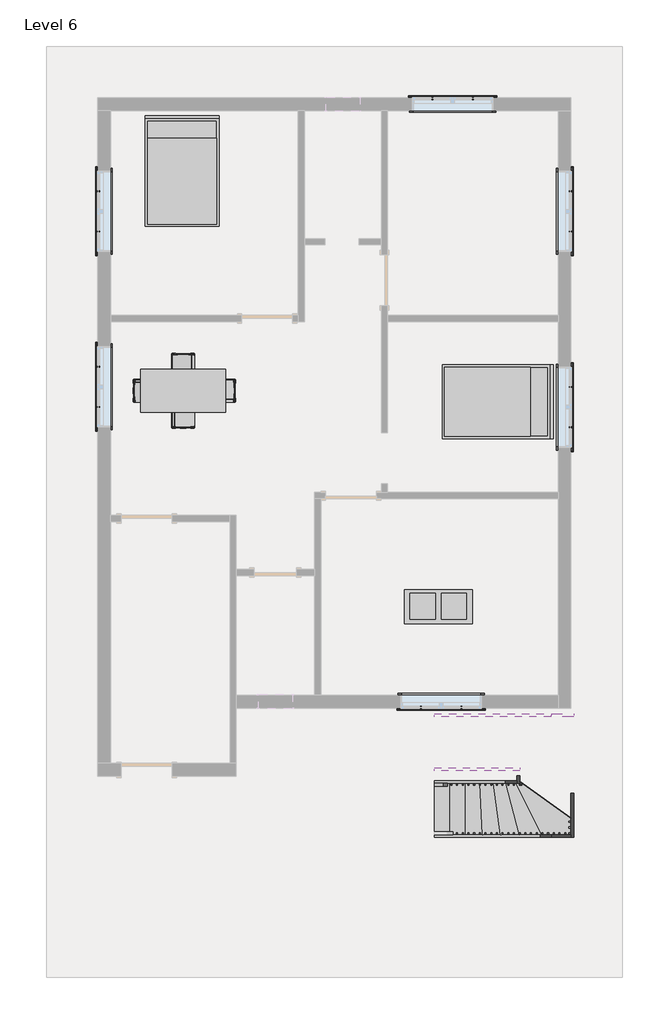
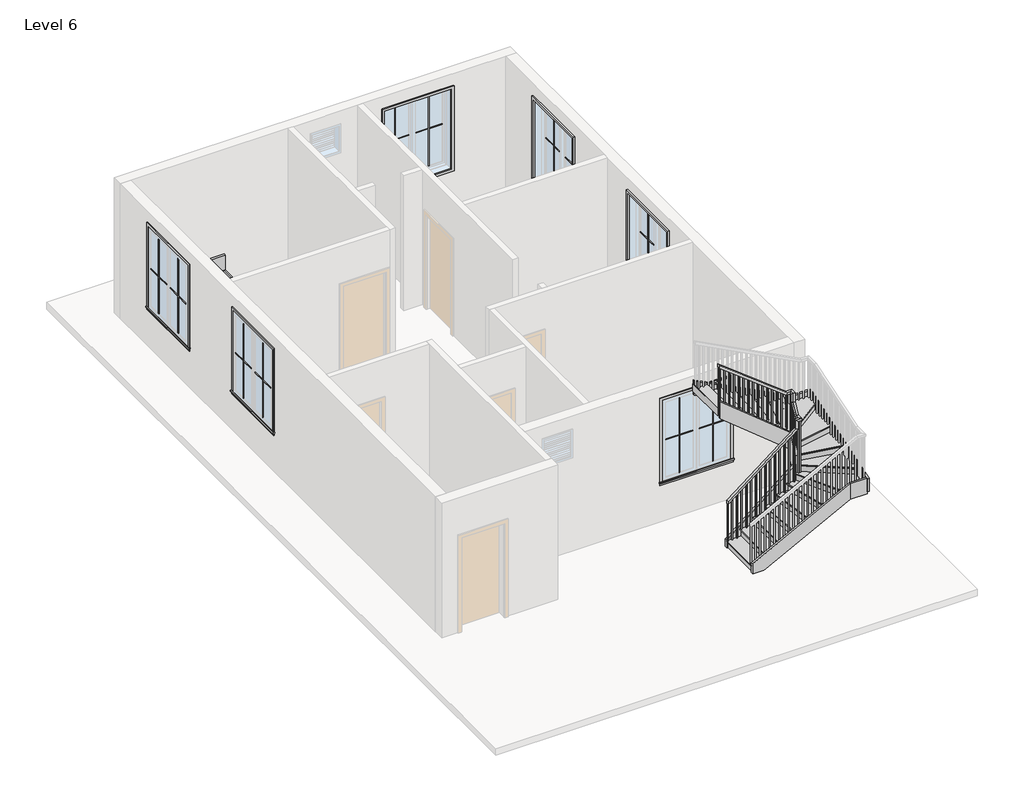
# One storey, part 3 of 3: 25 proxies, 8 members, 3 furniture elements, 1 railing, 1 stair flight.
"""IFC4 building model written with IfcOpenShell, lengths in millimetres."""

from ifc_helpers import new_model, si_unit, frame, origin, place, context, project, spatial, polyline, outline, extrude, faceted_brep, transform, mapped, element, save
from components import muntin_pattern_2x2_muntin_pattern_2x2_bff912c5, muntin_pattern_2x2_muntin_pattern_2x2_c2194282, trim_window_exterior_flat_with_sill_e04b3088, trim_window_interior_flat_picture_frame_2a7685fe, coffee_table_with_brass_mullions_11320_coffee_table_with_5962bef7, bed_17739_bed_17739_15c61121, dining_table_w_chairs_11374_0cdfc61b, stair_flight_916a27e3

model = new_model("IFC4")

# Units and contexts
model_context = context("Model", 3, world=origin())
ifc_project = project(units=[si_unit("LENGTHUNIT", "METRE", prefix="MILLI")], contexts=[model_context])

# Site, building, storey
site = spatial("IfcSite", under=ifc_project)
building = spatial("IfcBuilding", under=site)
storey = spatial("IfcBuildingStorey", under=building, Name="Level 6", Elevation=12801.6)

# Proxies
placement = place(None, origin())
muntin_pattern_2x2_muntin_pattern_2x2_shape = muntin_pattern_2x2_muntin_pattern_2x2_bff912c5(model_context)
element("IfcBuildingElementProxy", 1, Name="Muntin Pattern_2x2 : Muntin Pattern_2x2", ObjectType="Muntin Pattern_2x2 : Muntin Pattern_2x2", at=placement, inside=storey, context=model_context, shape_type="MappedRepresentation", body=[
    mapped(muntin_pattern_2x2_muntin_pattern_2x2_shape, transform((2964.3605034, 427.8534591, 13785.85), x_axis=(0.0, -1.0, 0.0), y_axis=(1.0, 0.0, 0.0), z_axis=(0.0, 0.0, 1.0))),
])
element("IfcBuildingElementProxy", 2, Name="Muntin Pattern_2x2 : Muntin Pattern_2x2", ObjectType="Muntin Pattern_2x2 : Muntin Pattern_2x2", at=placement, inside=storey, context=model_context, shape_type="MappedRepresentation", body=[
    mapped(muntin_pattern_2x2_muntin_pattern_2x2_shape, transform((2964.3605034, 3923.5284591, 13785.85), x_axis=(0.0, -1.0, 0.0), y_axis=(1.0, 0.0, 0.0), z_axis=(0.0, 0.0, 1.0))),
])
element("IfcBuildingElementProxy", 3, Name="Muntin Pattern_2x2 : Muntin Pattern_2x2", ObjectType="Muntin Pattern_2x2 : Muntin Pattern_2x2", at=placement, inside=storey, context=model_context, shape_type="MappedRepresentation", body=[
    mapped(muntin_pattern_2x2_muntin_pattern_2x2_shape, transform((498.9730034, 5582.4659591, 13785.85), x_axis=(1.0, 0.0, 0.0), y_axis=(0.0, 1.0, 0.0), z_axis=(0.0, 0.0, 1.0))),
])
element("IfcBuildingElementProxy", 4, Name="Muntin Pattern_2x2 : Muntin Pattern_2x2", ObjectType="Muntin Pattern_2x2 : Muntin Pattern_2x2", at=placement, inside=storey, context=model_context, shape_type="MappedRepresentation", body=[
    mapped(muntin_pattern_2x2_muntin_pattern_2x2_shape, transform((-5474.7894966, 3202.8034591, 13785.85), x_axis=(0.0, 1.0, 0.0), y_axis=(-1.0, 0.0, 0.0), z_axis=(0.0, 0.0, 1.0))),
])
element("IfcBuildingElementProxy", 5, Name="Muntin Pattern_2x2 : Muntin Pattern_2x2", ObjectType="Muntin Pattern_2x2 : Muntin Pattern_2x2", at=placement, inside=storey, context=model_context, shape_type="MappedRepresentation", body=[
    mapped(muntin_pattern_2x2_muntin_pattern_2x2_shape, transform((-5474.7894966, 69.0784591, 13785.85), x_axis=(0.0, 1.0, 0.0), y_axis=(-1.0, 0.0, 0.0), z_axis=(0.0, 0.0, 1.0))),
])
element("IfcBuildingElementProxy", 6, Name="Muntin Pattern_2x2 : Muntin Pattern_2x2", ObjectType="Muntin Pattern_2x2 : Muntin Pattern_2x2", at=placement, inside=storey, context=model_context, shape_type="MappedRepresentation", body=[
    mapped(muntin_pattern_2x2_muntin_pattern_2x2_shape, transform((1013.3230034, -5295.0840409, 13785.85), x_axis=(-1.0, 0.0, 0.0), y_axis=(0.0, -1.0, 0.0), z_axis=(0.0, 0.0, 1.0))),
])
muntin_pattern_2x2_muntin_pattern_2x2_2_shape = muntin_pattern_2x2_muntin_pattern_2x2_c2194282(model_context)
element("IfcBuildingElementProxy", 7, Name="Muntin Pattern_2x2 : Muntin Pattern_2x2", ObjectType="Muntin Pattern_2x2 : Muntin Pattern_2x2", at=placement, inside=storey, context=model_context, shape_type="MappedRepresentation", body=[
    mapped(muntin_pattern_2x2_muntin_pattern_2x2_2_shape, transform((2964.3605034, -292.8715409, 13785.85), x_axis=(0.0, 1.0, 0.0), y_axis=(-1.0, 0.0, 0.0), z_axis=(0.0, 0.0, 1.0))),
])
element("IfcBuildingElementProxy", 8, Name="Muntin Pattern_2x2 : Muntin Pattern_2x2", ObjectType="Muntin Pattern_2x2 : Muntin Pattern_2x2", at=placement, inside=storey, context=model_context, shape_type="MappedRepresentation", body=[
    mapped(muntin_pattern_2x2_muntin_pattern_2x2_2_shape, transform((2964.3605034, 3202.8034591, 13785.85), x_axis=(0.0, 1.0, 0.0), y_axis=(-1.0, 0.0, 0.0), z_axis=(0.0, 0.0, 1.0))),
])
element("IfcBuildingElementProxy", 9, Name="Muntin Pattern_2x2 : Muntin Pattern_2x2", ObjectType="Muntin Pattern_2x2 : Muntin Pattern_2x2", at=placement, inside=storey, context=model_context, shape_type="MappedRepresentation", body=[
    mapped(muntin_pattern_2x2_muntin_pattern_2x2_2_shape, transform((1219.6980034, 5582.4659591, 13785.85), x_axis=(-1.0, 0.0, 0.0), y_axis=(0.0, -1.0, 0.0), z_axis=(0.0, 0.0, 1.0))),
])
element("IfcBuildingElementProxy", 10, Name="Muntin Pattern_2x2 : Muntin Pattern_2x2", ObjectType="Muntin Pattern_2x2 : Muntin Pattern_2x2", at=placement, inside=storey, context=model_context, shape_type="MappedRepresentation", body=[
    mapped(muntin_pattern_2x2_muntin_pattern_2x2_2_shape, transform((-5474.7894966, 3923.5284591, 13785.85), x_axis=(0.0, -1.0, 0.0), y_axis=(1.0, 0.0, 0.0), z_axis=(0.0, 0.0, 1.0))),
])
element("IfcBuildingElementProxy", 11, Name="Muntin Pattern_2x2 : Muntin Pattern_2x2", ObjectType="Muntin Pattern_2x2 : Muntin Pattern_2x2", at=placement, inside=storey, context=model_context, shape_type="MappedRepresentation", body=[
    mapped(muntin_pattern_2x2_muntin_pattern_2x2_2_shape, transform((-5474.7894966, 789.8034591, 13785.85), x_axis=(0.0, -1.0, 0.0), y_axis=(1.0, 0.0, 0.0), z_axis=(0.0, 0.0, 1.0))),
])
element("IfcBuildingElementProxy", 12, Name="Muntin Pattern_2x2 : Muntin Pattern_2x2", ObjectType="Muntin Pattern_2x2 : Muntin Pattern_2x2", at=placement, inside=storey, context=model_context, shape_type="MappedRepresentation", body=[
    mapped(muntin_pattern_2x2_muntin_pattern_2x2_2_shape, transform((292.5980034, -5295.0840409, 13785.85), x_axis=(1.0, 0.0, 0.0), y_axis=(0.0, 1.0, 0.0), z_axis=(0.0, 0.0, 1.0))),
])
trim_window_exterior_flat_with_sill_shape = trim_window_exterior_flat_with_sill_e04b3088(model_context)
element("IfcBuildingElementProxy", 13, Name="Trim-Window-Exterior-Flat : with Sill", ObjectType="Trim-Window-Exterior-Flat : with Sill", at=placement, inside=storey, context=model_context, shape_type="MappedRepresentation", body=[
    mapped(trim_window_exterior_flat_with_sill_shape, transform((2973.8855034, 67.4909591, 15544.8), x_axis=(0.0, 1.0, 0.0), y_axis=(0.0, 0.0, 1.0), z_axis=(1.0, 0.0, 0.0))),
])
element("IfcBuildingElementProxy", 14, Name="Trim-Window-Exterior-Flat : with Sill", ObjectType="Trim-Window-Exterior-Flat : with Sill", at=placement, inside=storey, context=model_context, shape_type="MappedRepresentation", body=[
    mapped(trim_window_exterior_flat_with_sill_shape, transform((2973.8855034, 3563.1659591, 15544.8), x_axis=(0.0, 1.0, 0.0), y_axis=(0.0, 0.0, 1.0), z_axis=(1.0, 0.0, 0.0))),
])
element("IfcBuildingElementProxy", 15, Name="Trim-Window-Exterior-Flat : with Sill", ObjectType="Trim-Window-Exterior-Flat : with Sill", at=placement, inside=storey, context=model_context, shape_type="MappedRepresentation", body=[
    mapped(trim_window_exterior_flat_with_sill_shape, transform((859.3355034, 5591.9909591, 15544.8), x_axis=(-1.0, 0.0, 0.0), y_axis=(0.0, 0.0, 1.0), z_axis=(0.0, 1.0, 0.0))),
])
element("IfcBuildingElementProxy", 16, Name="Trim-Window-Exterior-Flat : with Sill", ObjectType="Trim-Window-Exterior-Flat : with Sill", at=placement, inside=storey, context=model_context, shape_type="MappedRepresentation", body=[
    mapped(trim_window_exterior_flat_with_sill_shape, transform((-5484.3144966, 3563.1659591, 15544.8), x_axis=(0.0, -1.0, 0.0), y_axis=(0.0, 0.0, 1.0), z_axis=(-1.0, 0.0, 0.0))),
])
element("IfcBuildingElementProxy", 17, Name="Trim-Window-Exterior-Flat : with Sill", ObjectType="Trim-Window-Exterior-Flat : with Sill", at=placement, inside=storey, context=model_context, shape_type="MappedRepresentation", body=[
    mapped(trim_window_exterior_flat_with_sill_shape, transform((-5484.3144966, 429.4409591, 15544.8), x_axis=(0.0, -1.0, 0.0), y_axis=(0.0, 0.0, 1.0), z_axis=(-1.0, 0.0, 0.0))),
])
element("IfcBuildingElementProxy", 18, Name="Trim-Window-Exterior-Flat : with Sill", ObjectType="Trim-Window-Exterior-Flat : with Sill", at=placement, inside=storey, context=model_context, shape_type="MappedRepresentation", body=[
    mapped(trim_window_exterior_flat_with_sill_shape, transform((652.9605034, -5304.6090409, 15544.8), x_axis=(1.0, 0.0, 0.0), y_axis=(0.0, 0.0, 1.0), z_axis=(0.0, -1.0, 0.0))),
])
trim_window_interior_flat_picture_frame_shape = trim_window_interior_flat_picture_frame_2a7685fe(model_context)
element("IfcBuildingElementProxy", 19, Name="Trim-Window-Interior-Flat : Picture Frame", ObjectType="Trim-Window-Interior-Flat : Picture Frame", at=placement, inside=storey, context=model_context, shape_type="MappedRepresentation", body=[
    mapped(trim_window_interior_flat_picture_frame_shape, transform((2745.2855034, 67.4909591, 15544.8), x_axis=(0.0, -1.0, 0.0), y_axis=(0.0, 0.0, 1.0), z_axis=(-1.0, 0.0, 0.0))),
])
element("IfcBuildingElementProxy", 20, Name="Trim-Window-Interior-Flat : Picture Frame", ObjectType="Trim-Window-Interior-Flat : Picture Frame", at=placement, inside=storey, context=model_context, shape_type="MappedRepresentation", body=[
    mapped(trim_window_interior_flat_picture_frame_shape, transform((2745.2855034, 3563.1659591, 15544.8), x_axis=(0.0, -1.0, 0.0), y_axis=(0.0, 0.0, 1.0), z_axis=(-1.0, 0.0, 0.0))),
])
element("IfcBuildingElementProxy", 21, Name="Trim-Window-Interior-Flat : Picture Frame", ObjectType="Trim-Window-Interior-Flat : Picture Frame", at=placement, inside=storey, context=model_context, shape_type="MappedRepresentation", body=[
    mapped(trim_window_interior_flat_picture_frame_shape, transform((859.3355034, 5363.3909591, 15544.8), x_axis=(1.0, 0.0, 0.0), y_axis=(0.0, 0.0, 1.0), z_axis=(0.0, -1.0, 0.0))),
])
element("IfcBuildingElementProxy", 22, Name="Trim-Window-Interior-Flat : Picture Frame", ObjectType="Trim-Window-Interior-Flat : Picture Frame", at=placement, inside=storey, context=model_context, shape_type="MappedRepresentation", body=[
    mapped(trim_window_interior_flat_picture_frame_shape, transform((-5255.7144966, 3563.1659591, 15544.8), x_axis=(0.0, 1.0, 0.0), y_axis=(0.0, 0.0, 1.0), z_axis=(1.0, 0.0, 0.0))),
])
element("IfcBuildingElementProxy", 23, Name="Trim-Window-Interior-Flat : Picture Frame", ObjectType="Trim-Window-Interior-Flat : Picture Frame", at=placement, inside=storey, context=model_context, shape_type="MappedRepresentation", body=[
    mapped(trim_window_interior_flat_picture_frame_shape, transform((-5255.7144966, 429.4409591, 15544.8), x_axis=(0.0, 1.0, 0.0), y_axis=(0.0, 0.0, 1.0), z_axis=(1.0, 0.0, 0.0))),
])
element("IfcBuildingElementProxy", 24, Name="Trim-Window-Interior-Flat : Picture Frame", ObjectType="Trim-Window-Interior-Flat : Picture Frame", at=placement, inside=storey, context=model_context, shape_type="MappedRepresentation", body=[
    mapped(trim_window_interior_flat_picture_frame_shape, transform((652.9605034, -5076.0090409, 15544.8), x_axis=(-1.0, 0.0, 0.0), y_axis=(0.0, 0.0, 1.0), z_axis=(0.0, 1.0, 0.0))),
])
coffee_table_with_brass_mullions_11320_coffee_table_with_shape = coffee_table_with_brass_mullions_11320_coffee_table_with_5962bef7(model_context)
element("IfcBuildingElementProxy", 25, Name="coffee_table_with_brass_mullions_11320 : coffee_table_with_brass_mullions_11320", ObjectType="coffee_table_with_brass_mullions_11320 : coffee_table_with_brass_mullions_11320", at=placement, inside=storey, context=model_context, shape_type="MappedRepresentation", body=[
    mapped(coffee_table_with_brass_mullions_11320_coffee_table_with_shape, transform((1240.0943553, -3926.0808329, 12801.6), x_axis=(1.0, 0.0, 0.0), y_axis=(0.0, 1.0, 0.0), z_axis=(0.0, 0.0, 1.0))),
])

# Furniture
bed_17739_bed_17739_shape = bed_17739_bed_17739_15c61121(model_context)
element("IfcFurniture", 26, ObjectType="Bed_17739 : Bed_17739", at=placement, inside=storey, context=model_context, shape_type="MappedRepresentation", body=[
    mapped(bed_17739_bed_17739_shape, transform((-3979.3644966, 4258.4909591, 12801.6), x_axis=(1.0, 0.0, 0.0), y_axis=(0.0, 1.0, 0.0), z_axis=(0.0, 0.0, 1.0))),
])
element("IfcFurniture", 27, ObjectType="Bed_17739 : Bed_17739", at=placement, inside=storey, context=model_context, shape_type="MappedRepresentation", body=[
    mapped(bed_17739_bed_17739_shape, transform((1640.3855034, 162.7409591, 12801.6), x_axis=(0.0, -1.0, 0.0), y_axis=(1.0, 0.0, 0.0), z_axis=(0.0, 0.0, 1.0))),
])
dining_table_w_chairs_11374_shape = dining_table_w_chairs_11374_0cdfc61b(model_context)
element("IfcFurniture", 28, ObjectType="Dining_Table_w_Chairs_11374", at=placement, inside=storey, context=model_context, shape_type="MappedRepresentation", body=[
    mapped(dining_table_w_chairs_11374_shape, transform((-3975.2132663, 265.1952874, 12801.6), x_axis=(1.0, 0.0, 0.0), y_axis=(0.0, 1.0, 0.0), z_axis=(0.0, 0.0, 1.0))),
])

# Members
element("IfcMember", 29, ObjectType="Stringer - 2\" Width", at=placement, inside=storey, context=model_context, shape_type="SweptSolid", body=[
    extrude(outline(polyline([(12977.7764461, 531.7538115), (12801.6, 531.7538115), (12801.6, 798.0154561), (13788.7410923, 2008.6855034), (14182.018648, 2008.6855034), (12977.7764461, 531.7538115)])), frame((0.0, -6650.8090409, 0.0), z_axis=(0.0, 1.0, 0.0), x_axis=(0.0, 0.0, 1.0)), (0.0, 0.0, 1.0), 50.8),
])
element("IfcMember", 30, ObjectType="Stringer - 2\" Width", at=placement, inside=storey, context=model_context, shape_type="SweptSolid", body=[
    extrude(outline(polyline([(-6650.8090409, 13830.1617647), (-6650.8090409, 14374.8682978), (-6444.1719234, 14727.7409689), (-6422.2090409, 14727.7409689), (-6422.2090409, 14162.065107), (-6616.5668235, 13830.1617647), (-6650.8090409, 13830.1617647)])), frame((2008.6855034, 0.0, 0.0), z_axis=(1.0, 0.0, 0.0), x_axis=(0.0, 1.0, 0.0)), (0.0, 0.0, 1.0), 50.8),
])
element("IfcMember", 31, ObjectType="Stringer - 2\" Width", at=placement, inside=storey, context=model_context, shape_type="SweptSolid", body=[
    extrude(outline(polyline([(14334.4634131, 2059.4855034), (14727.7409689, 2059.4855034), (15973.4038432, 531.7538115), (15580.1262875, 531.7538115), (14334.4634131, 2059.4855034)])), frame((0.0, -6422.2090409, 0.0), z_axis=(0.0, 1.0, 0.0), x_axis=(0.0, 0.0, 1.0)), (0.0, 0.0, 1.0), 50.8),
])
element("IfcMember", 32, ObjectType="Stringer - 2\" Width", at=placement, inside=storey, context=model_context, shape_type="SweptSolid", body=[
    extrude(outline(polyline([(13031.239954, 531.7538115), (12801.6, 531.7538115), (12801.6, 751.5161291), (13764.100629, 2619.1710032), (14106.9956453, 2619.1710032), (13031.239954, 531.7538115)])), frame((0.0, -7616.0090409, 0.0), z_axis=(0.0, 1.0, 0.0), x_axis=(0.0, 0.0, 1.0)), (0.0, 0.0, 1.0), 50.8),
])
element("IfcMember", 33, ObjectType="Stringer - 2\" Width", at=placement, inside=storey, context=model_context, shape_type="SweptSolid", body=[
    extrude(outline(polyline([(2619.1710032, -7616.0090409), (2619.1710032, -7565.2090409), (2973.8855034, -7565.2090409), (2973.8855034, -7616.0090409), (2619.1710032, -7616.0090409)])), frame((0.0, 0.0, 13764.100629), z_axis=(0.0, 0.0, 1.0), x_axis=(1.0, 0.0, 0.0)), (0.0, 0.0, 1.0), 342.8950162),
])
element("IfcMember", 34, ObjectType="Stringer - 2\" Width", at=placement, inside=storey, context=model_context, shape_type="SweptSolid", body=[
    extrude(outline(polyline([(-7616.0090409, 13802.1956453), (-7616.0090409, 14090.6952212), (-5493.9891581, 14771.5972697), (-5457.0090409, 14771.5972697), (-5457.0090409, 14440.5682298), (-7446.4865579, 13802.1956453), (-7616.0090409, 13802.1956453)])), frame((2973.8855034, 0.0, 0.0), z_axis=(1.0, 0.0, 0.0), x_axis=(0.0, 1.0, 0.0)), (0.0, 0.0, 1.0), 50.8),
])
element("IfcMember", 35, ObjectType="Stringer - 2\" Width", at=placement, inside=storey, context=model_context, shape_type="SweptSolid", body=[
    extrude(outline(polyline([(3024.6855034, -5406.2090409), (3024.6855034, -5457.0090409), (2619.1710032, -5457.0090409), (2619.1710032, -5406.2090409), (3024.6855034, -5406.2090409)])), frame((0.0, 0.0, 14451.4904473), z_axis=(0.0, 0.0, 1.0), x_axis=(1.0, 0.0, 0.0)), (0.0, 0.0, 1.0), 320.1068224),
])
element("IfcMember", 36, ObjectType="Stringer - 2\" Width", at=placement, inside=storey, context=model_context, shape_type="SweptSolid", body=[
    extrude(outline(polyline([(14451.4904473, 2619.1710032), (14771.5972697, 2619.1710032), (15847.3529609, 531.7538115), (15527.2461385, 531.7538115), (14451.4904473, 2619.1710032)])), frame((0.0, -5457.0090409, 0.0), z_axis=(0.0, 1.0, 0.0), x_axis=(0.0, 0.0, 1.0)), (0.0, 0.0, 1.0), 50.8),
])

# Railing
element("IfcRailing", 37, ObjectType="Handrail - Rectangular", at=placement, inside=storey, context=model_context, shape_type="SolidModel", body=[
    faceted_brep([(531.7538115, -6650.8090409, 13885.3333333), (531.7538115, -6650.8090409, 13821.0000346), (531.7538115, -6701.6090409, 13821.0000346), (531.7538115, -6701.6090409, 13885.3333333), (1983.2855034, -6650.8090409, 15013.2191036), (2034.0855034, -6650.8090409, 14988.3590024), (2034.0855034, -6701.6090409, 14988.3590024), (1983.2855034, -6701.6090409, 15013.2191036), (2059.4855034, -6545.487707, 15165.4281882), (2059.4855034, -6574.6090409, 15216.2281882), (2059.4855034, -6447.6090409, 15433.1051451), (2059.4855034, -6396.8090409, 15419.3256424), (2110.2855034, -6545.487707, 15165.4281882), (2110.2855034, -6396.8090409, 15419.3256424), (2110.2855034, -6574.6090409, 15216.2281882), (2110.2855034, -6447.6090409, 15433.1051451), (531.7538115, -6371.4090409, 16764.0), (531.7538115, -6320.6090409, 16764.0), (531.7538115, -6320.6090409, 16699.6667013), (531.7538115, -6371.4090409, 16699.6667013), (1965.8688354, -6371.4090409, 15585.3142297), (1983.2855034, -6371.4090409, 15636.1142297), (1965.8688354, -6320.6090409, 15585.3142297), (1983.2855034, -6320.6090409, 15636.1142297), (1983.2855034, -6650.8090409, 15216.2281882), (2034.0855034, -6650.8090409, 15165.4281882), (2034.0855034, -6701.6090409, 15165.4281882), (1983.2855034, -6701.6090409, 15216.2281882), (2059.4855034, -6650.8090409, 15216.2281882), (2059.4855034, -6650.8090409, 15165.4281882), (2110.2855034, -6701.6090409, 15165.4281882), (2110.2855034, -6701.6090409, 15216.2281882), (2059.4855034, -6447.6090409, 15636.1142297), (2059.4855034, -6396.8090409, 15585.3142297), (2110.2855034, -6396.8090409, 15585.3142297), (2110.2855034, -6447.6090409, 15636.1142297), (2059.4855034, -6371.4090409, 15636.1142297), (2059.4855034, -6371.4090409, 15585.3142297), (2110.2855034, -6320.6090409, 15585.3142297), (2110.2855034, -6320.6090409, 15636.1142297)], [[[0, 1, 2, 3]], [[1, 0, 4, 5]], [[2, 1, 5, 6]], [[3, 2, 6, 7]], [[0, 3, 7, 4]], [[8, 9, 10, 11]], [[12, 8, 11, 13]], [[14, 12, 13, 15]], [[9, 14, 15, 10]], [[16, 17, 18, 19]], [[20, 21, 16, 19]], [[22, 20, 19, 18]], [[23, 22, 18, 17]], [[21, 23, 17, 16]], [[5, 4, 24, 25]], [[6, 5, 25, 26]], [[7, 6, 26, 27]], [[4, 7, 27, 24]], [[25, 24, 28, 29]], [[26, 25, 29, 30]], [[27, 26, 30, 31]], [[24, 27, 31, 28]], [[29, 28, 9, 8]], [[30, 29, 8, 12]], [[31, 30, 12, 14]], [[28, 31, 14, 9]], [[11, 10, 32, 33]], [[13, 11, 33, 34]], [[15, 13, 34, 35]], [[10, 15, 35, 32]], [[33, 32, 36, 37]], [[34, 33, 37, 38]], [[35, 34, 38, 39]], [[32, 35, 39, 36]], [[37, 36, 21, 20]], [[38, 37, 20, 22]], [[39, 38, 22, 23]], [[36, 39, 23, 21]]]),
    extrude(outline(polyline([(16684.4316852, 551.3605034), (15680.2666667, 551.3605034), (15680.2666667, 570.4105034), (16669.6292361, 570.4105034), (16684.4316852, 551.3605034)])), frame((0.0, -6355.5340409, 0.0), z_axis=(0.0, 1.0, 0.0), x_axis=(0.0, 0.0, 1.0)), (0.0, 0.0, 1.0), 19.05),
    extrude(outline(polyline([(16605.4852902, 652.9605034), (15680.2666667, 652.9605034), (15680.2666667, 672.0105034), (16590.6828411, 672.0105034), (16605.4852902, 652.9605034)])), frame((0.0, -6355.5340409, 0.0), z_axis=(0.0, 1.0, 0.0), x_axis=(0.0, 0.0, 1.0)), (0.0, 0.0, 1.0), 19.05),
    extrude(outline(polyline([(16526.5388952, 754.5605034), (15680.2666667, 754.5605034), (15680.2666667, 773.6105034), (16511.7364462, 773.6105034), (16526.5388952, 754.5605034)])), frame((0.0, -6355.5340409, 0.0), z_axis=(0.0, 1.0, 0.0), x_axis=(0.0, 0.0, 1.0)), (0.0, 0.0, 1.0), 19.05),
    extrude(outline(polyline([(16447.5925003, 856.1605034), (15510.9333333, 856.1605034), (15510.9333333, 875.2105034), (16432.7900512, 875.2105034), (16447.5925003, 856.1605034)])), frame((0.0, -6355.5340409, 0.0), z_axis=(0.0, 1.0, 0.0), x_axis=(0.0, 0.0, 1.0)), (0.0, 0.0, 1.0), 19.05),
    extrude(outline(polyline([(16368.6461053, 957.7605034), (15510.9333333, 957.7605034), (15510.9333333, 976.8105034), (16353.8436562, 976.8105034), (16368.6461053, 957.7605034)])), frame((0.0, -6355.5340409, 0.0), z_axis=(0.0, 1.0, 0.0), x_axis=(0.0, 0.0, 1.0)), (0.0, 0.0, 1.0), 19.05),
    extrude(outline(polyline([(16289.6997103, 1059.3605034), (15510.9333333, 1059.3605034), (15510.9333333, 1078.4105034), (16274.8972613, 1078.4105034), (16289.6997103, 1059.3605034)])), frame((0.0, -6355.5340409, 0.0), z_axis=(0.0, 1.0, 0.0), x_axis=(0.0, 0.0, 1.0)), (0.0, 0.0, 1.0), 19.05),
    extrude(outline(polyline([(16210.7533154, 1160.9605034), (15341.6, 1160.9605034), (15341.6, 1180.0105034), (16195.9508663, 1180.0105034), (16210.7533154, 1160.9605034)])), frame((0.0, -6355.5340409, 0.0), z_axis=(0.0, 1.0, 0.0), x_axis=(0.0, 0.0, 1.0)), (0.0, 0.0, 1.0), 19.05),
    extrude(outline(polyline([(16131.8069204, 1262.5605034), (15341.6, 1262.5605034), (15341.6, 1281.6105034), (16117.0044713, 1281.6105034), (16131.8069204, 1262.5605034)])), frame((0.0, -6355.5340409, 0.0), z_axis=(0.0, 1.0, 0.0), x_axis=(0.0, 0.0, 1.0)), (0.0, 0.0, 1.0), 19.05),
    extrude(outline(polyline([(16052.8605254, 1364.1605034), (15172.2666667, 1364.1605034), (15172.2666667, 1383.2105034), (16038.0580764, 1383.2105034), (16052.8605254, 1364.1605034)])), frame((0.0, -6355.5340409, 0.0), z_axis=(0.0, 1.0, 0.0), x_axis=(0.0, 0.0, 1.0)), (0.0, 0.0, 1.0), 19.05),
    extrude(outline(polyline([(15973.9141304, 1465.7605034), (15172.2666667, 1465.7605034), (15172.2666667, 1484.8105034), (15959.1116814, 1484.8105034), (15973.9141304, 1465.7605034)])), frame((0.0, -6355.5340409, 0.0), z_axis=(0.0, 1.0, 0.0), x_axis=(0.0, 0.0, 1.0)), (0.0, 0.0, 1.0), 19.05),
    extrude(outline(polyline([(15894.9677355, 1567.3605034), (15172.2666667, 1567.3605034), (15172.2666667, 1586.4105034), (15880.1652864, 1586.4105034), (15894.9677355, 1567.3605034)])), frame((0.0, -6355.5340409, 0.0), z_axis=(0.0, 1.0, 0.0), x_axis=(0.0, 0.0, 1.0)), (0.0, 0.0, 1.0), 19.05),
    extrude(outline(polyline([(15816.0213405, 1668.9605034), (15002.9333333, 1668.9605034), (15002.9333333, 1688.0105034), (15801.2188914, 1688.0105034), (15816.0213405, 1668.9605034)])), frame((0.0, -6355.5340409, 0.0), z_axis=(0.0, 1.0, 0.0), x_axis=(0.0, 0.0, 1.0)), (0.0, 0.0, 1.0), 19.05),
    extrude(outline(polyline([(15737.0749455, 1770.5605034), (15002.9333333, 1770.5605034), (15002.9333333, 1789.6105034), (15722.2724965, 1789.6105034), (15737.0749455, 1770.5605034)])), frame((0.0, -6355.5340409, 0.0), z_axis=(0.0, 1.0, 0.0), x_axis=(0.0, 0.0, 1.0)), (0.0, 0.0, 1.0), 19.05),
    extrude(outline(polyline([(15658.1285506, 1872.1605034), (14833.6, 1872.1605034), (14833.6, 1891.2105034), (15643.3261015, 1891.2105034), (15658.1285506, 1872.1605034)])), frame((0.0, -6355.5340409, 0.0), z_axis=(0.0, 1.0, 0.0), x_axis=(0.0, 0.0, 1.0)), (0.0, 0.0, 1.0), 19.05),
    extrude(outline(polyline([(15579.1821556, 1973.7605034), (14833.6, 1973.7605034), (14833.6, 1992.8105034), (15564.3797065, 1992.8105034), (15579.1821556, 1973.7605034)])), frame((0.0, -6355.5340409, 0.0), z_axis=(0.0, 1.0, 0.0), x_axis=(0.0, 0.0, 1.0)), (0.0, 0.0, 1.0), 19.05),
    extrude(outline(polyline([(2075.3605034, -6380.9340409), (2075.3605034, -6361.8840409), (2094.4105034, -6361.8840409), (2094.4105034, -6380.9340409), (2075.3605034, -6380.9340409)])), frame((0.0, 0.0, 14494.9333333), z_axis=(0.0, 0.0, 1.0), x_axis=(1.0, 0.0, 0.0)), (0.0, 0.0, 1.0), 1090.3808964),
    extrude(outline(polyline([(-6463.4840409, 15305.46524), (-6463.4840409, 14325.6), (-6482.5340409, 14325.6), (-6482.5340409, 15272.9336964), (-6463.4840409, 15305.46524)])), frame((2075.3605034, 0.0, 0.0), z_axis=(1.0, 0.0, 0.0), x_axis=(0.0, 1.0, 0.0)), (0.0, 0.0, 1.0), 19.05),
    extrude(outline(polyline([(-6565.0840409, 15131.9636744), (-6565.0840409, 14156.2666667), (-6584.1340409, 14156.2666667), (-6584.1340409, 15099.4321309), (-6565.0840409, 15131.9636744)])), frame((2075.3605034, 0.0, 0.0), z_axis=(1.0, 0.0, 0.0), x_axis=(0.0, 1.0, 0.0)), (0.0, 0.0, 1.0), 19.05),
    extrude(outline(polyline([(2046.2288115, -6666.6840409), (2065.2788115, -6666.6840409), (2065.2788115, -6685.7340409), (2046.2288115, -6685.7340409), (2046.2288115, -6666.6840409)])), frame((0.0, 0.0, 13986.9333333), z_axis=(0.0, 0.0, 1.0), x_axis=(1.0, 0.0, 0.0)), (0.0, 0.0, 1.0), 1178.4948549),
    extrude(outline(polyline([(14918.8483397, 1944.6288115), (13817.6, 1944.6288115), (13817.6, 1963.6788115), (14933.6507888, 1963.6788115), (14918.8483397, 1944.6288115)])), frame((0.0, -6685.7340409, 0.0), z_axis=(0.0, 1.0, 0.0), x_axis=(0.0, 0.0, 1.0)), (0.0, 0.0, 1.0), 19.05),
    extrude(outline(polyline([(14839.9019447, 1843.0288115), (13817.6, 1843.0288115), (13817.6, 1862.0788115), (14854.7043938, 1862.0788115), (14839.9019447, 1843.0288115)])), frame((0.0, -6685.7340409, 0.0), z_axis=(0.0, 1.0, 0.0), x_axis=(0.0, 0.0, 1.0)), (0.0, 0.0, 1.0), 19.05),
    extrude(outline(polyline([(14760.9555498, 1741.4288115), (13648.2666667, 1741.4288115), (13648.2666667, 1760.4788115), (14775.7579988, 1760.4788115), (14760.9555498, 1741.4288115)])), frame((0.0, -6685.7340409, 0.0), z_axis=(0.0, 1.0, 0.0), x_axis=(0.0, 0.0, 1.0)), (0.0, 0.0, 1.0), 19.05),
    extrude(outline(polyline([(14682.0091548, 1639.8288115), (13648.2666667, 1639.8288115), (13648.2666667, 1658.8788115), (14696.8116039, 1658.8788115), (14682.0091548, 1639.8288115)])), frame((0.0, -6685.7340409, 0.0), z_axis=(0.0, 1.0, 0.0), x_axis=(0.0, 0.0, 1.0)), (0.0, 0.0, 1.0), 19.05),
    extrude(outline(polyline([(14603.0627598, 1538.2288115), (13478.9333333, 1538.2288115), (13478.9333333, 1557.2788115), (14617.8652089, 1557.2788115), (14603.0627598, 1538.2288115)])), frame((0.0, -6685.7340409, 0.0), z_axis=(0.0, 1.0, 0.0), x_axis=(0.0, 0.0, 1.0)), (0.0, 0.0, 1.0), 19.05),
    extrude(outline(polyline([(14524.1163649, 1436.6288115), (13478.9333333, 1436.6288115), (13478.9333333, 1455.6788115), (14538.9188139, 1455.6788115), (14524.1163649, 1436.6288115)])), frame((0.0, -6685.7340409, 0.0), z_axis=(0.0, 1.0, 0.0), x_axis=(0.0, 0.0, 1.0)), (0.0, 0.0, 1.0), 19.05),
    extrude(outline(polyline([(14445.1699699, 1335.0288115), (13309.6, 1335.0288115), (13309.6, 1354.0788115), (14459.9724189, 1354.0788115), (14445.1699699, 1335.0288115)])), frame((0.0, -6685.7340409, 0.0), z_axis=(0.0, 1.0, 0.0), x_axis=(0.0, 0.0, 1.0)), (0.0, 0.0, 1.0), 19.05),
    extrude(outline(polyline([(14366.2235749, 1233.4288115), (13309.6, 1233.4288115), (13309.6, 1252.4788115), (14381.026024, 1252.4788115), (14366.2235749, 1233.4288115)])), frame((0.0, -6685.7340409, 0.0), z_axis=(0.0, 1.0, 0.0), x_axis=(0.0, 0.0, 1.0)), (0.0, 0.0, 1.0), 19.05),
    extrude(outline(polyline([(14287.2771799, 1131.8288115), (13309.6, 1131.8288115), (13309.6, 1150.8788115), (14302.079629, 1150.8788115), (14287.2771799, 1131.8288115)])), frame((0.0, -6685.7340409, 0.0), z_axis=(0.0, 1.0, 0.0), x_axis=(0.0, 0.0, 1.0)), (0.0, 0.0, 1.0), 19.05),
    extrude(outline(polyline([(14208.330785, 1030.2288115), (13140.2666667, 1030.2288115), (13140.2666667, 1049.2788115), (14223.133234, 1049.2788115), (14208.330785, 1030.2288115)])), frame((0.0, -6685.7340409, 0.0), z_axis=(0.0, 1.0, 0.0), x_axis=(0.0, 0.0, 1.0)), (0.0, 0.0, 1.0), 19.05),
    extrude(outline(polyline([(14129.38439, 928.6288115), (13140.2666667, 928.6288115), (13140.2666667, 947.6788115), (14144.1868391, 947.6788115), (14129.38439, 928.6288115)])), frame((0.0, -6685.7340409, 0.0), z_axis=(0.0, 1.0, 0.0), x_axis=(0.0, 0.0, 1.0)), (0.0, 0.0, 1.0), 19.05),
    extrude(outline(polyline([(14050.437995, 827.0288115), (13140.2666667, 827.0288115), (13140.2666667, 846.0788115), (14065.2404441, 846.0788115), (14050.437995, 827.0288115)])), frame((0.0, -6685.7340409, 0.0), z_axis=(0.0, 1.0, 0.0), x_axis=(0.0, 0.0, 1.0)), (0.0, 0.0, 1.0), 19.05),
    extrude(outline(polyline([(13971.4916001, 725.4288115), (12970.9333333, 725.4288115), (12970.9333333, 744.4788115), (13986.2940491, 744.4788115), (13971.4916001, 725.4288115)])), frame((0.0, -6685.7340409, 0.0), z_axis=(0.0, 1.0, 0.0), x_axis=(0.0, 0.0, 1.0)), (0.0, 0.0, 1.0), 19.05),
    extrude(outline(polyline([(13892.5452051, 623.8288115), (12970.9333333, 623.8288115), (12970.9333333, 642.8788115), (13907.3476541, 642.8788115), (13892.5452051, 623.8288115)])), frame((0.0, -6685.7340409, 0.0), z_axis=(0.0, 1.0, 0.0), x_axis=(0.0, 0.0, 1.0)), (0.0, 0.0, 1.0), 19.05),
    extrude(outline(polyline([(2075.3605034, -6355.5340409), (2075.3605034, -6336.4840409), (2094.4105034, -6336.4840409), (2094.4105034, -6355.5340409), (2075.3605034, -6355.5340409)])), frame((0.0, 0.0, 14664.2666667), z_axis=(0.0, 0.0, 1.0), x_axis=(1.0, 0.0, 0.0)), (0.0, 0.0, 1.0), 921.0475631),
    extrude(outline(polyline([(2075.3605034, -6666.6840409), (2094.4105034, -6666.6840409), (2094.4105034, -6685.7340409), (2075.3605034, -6685.7340409), (2075.3605034, -6666.6840409)])), frame((0.0, 0.0, 13986.9333333), z_axis=(0.0, 0.0, 1.0), x_axis=(1.0, 0.0, 0.0)), (0.0, 0.0, 1.0), 1178.4948549),
    extrude(outline(polyline([(16699.6667013, 531.7538115), (15680.2666667, 531.7538115), (15680.2666667, 550.8038115), (16684.8642523, 550.8038115), (16699.6667013, 531.7538115)])), frame((0.0, -6355.5340409, 0.0), z_axis=(0.0, 1.0, 0.0), x_axis=(0.0, 0.0, 1.0)), (0.0, 0.0, 1.0), 19.05),
    extrude(outline(polyline([(13821.0000346, 531.7538115), (12970.9333333, 531.7538115), (12970.9333333, 550.8038115), (13835.8024837, 550.8038115), (13821.0000346, 531.7538115)])), frame((0.0, -6685.7340409, 0.0), z_axis=(0.0, 1.0, 0.0), x_axis=(0.0, 0.0, 1.0)), (0.0, 0.0, 1.0), 19.05),
])

# Stair flight
stair_flight_shape = stair_flight_916a27e3(model_context)
element("IfcStairFlight", 38, ObjectType="2\" Tread 1\" Nosing 1/4\" Riser", at=placement, inside=storey, context=model_context, shape_type="MappedRepresentation", body=[
    mapped(stair_flight_shape, transform((0.0, 0.0, 0.0), x_axis=(1.0, 0.0, 0.0), y_axis=(0.0, 1.0, 0.0), z_axis=(0.0, 0.0, 1.0))),
])

save(model, "model.ifc")

# Revit data of these elements
# Type "Muntin Pattern_2x2 : Muntin Pattern_2x2"
#   Width [instance default] = 4' - 0"
#   Thickness = 0' - 0 1/2"
#   Height [instance default] = 4' - 0"
#   Distance = 0' - 0 3/4"
#   Interior Material [instance default] = none
#   Exterior Material [instance default] = none
#   Default Elevation = 0
# Type "Trim-Window-Exterior-Flat : with Sill"
#   Trim Width = 0' - 2 1/4"
#   Trim Thickness_Picture Frame = 0' - 1 1/4"
#   Trim Thickness_with Sill = 0' - 0 3/4"
#   Sill Thickness = 0' - 1 1/4"
#   Opening Width [instance default] = 2' - 0"
#   Opening Height [instance default] = 3' - 0"
#   Default Elevation = 4' - 0"
#   Sill = yes
#   Picture Frame = no
#   Trim Material [instance default] = none
# Type "Trim-Window-Interior-Flat : Picture Frame"
#   Trim Thickness_Picture Frame = 0' - 1 1/4"
#   Trim Width = 0' - 2 1/4"
#   Trim Thickness_with Sill = 0' - 0 3/4"
#   Sill Thickness = 0' - 1 1/4"
#   Opening Width [instance default] = 2' - 0"
#   Opening Height [instance default] = 3' - 0"
#   Default Elevation = 4' - 0"
#   Sill = no
#   Picture Frame = yes
#   Trim Material [instance default] = none
# Type "coffee_table_with_brass_mullions_11320 : coffee_table_with_brass_mullions_11320"
#   Default Elevation = 0
# Type "Bed_17739 : Bed_17739"
#   Default Elevation = 0
# Type "Dining_Table_w_Chairs_11374"
#   Default Elevation = 0
#   Assembly Code = ""
# Type "Handrail - Rectangular"
#   Assembly Code = "C2010400"
#   built-in parameter 1008612 = 0.0416667 (stored number, unit not read)
#   built-in parameter 1008611 = 0.0416667 (stored number, unit not read)
#   built-in parameter 1008609 = 0.333333 (stored number, unit not read)
#   built-in parameter 1008604 = 0.166667 (stored number, unit not read)
#   built-in parameter 1008603 = 0.166667 (stored number, unit not read)
#   Railing Height = 3' - 0"
#   built-in parameter 1008630 = 2
#   built-in parameter 1008610 = 2
#   built-in parameter 1008618 = Baluster - Square : 3/4"
# Elements 1, 2, 3, 4, 5, 6, 7, 8, 9, 10, 11, 12 (IfcBuildingElementProxy, "Muntin Pattern_2x2 : Muntin Pattern_2x2")
#   Width = 1' - 11 1/8"
#   Height = 5' - 6 1/2"
#   Interior Material = Wood - Stained
#   Exterior Material = Clad - White
#   Phase Created = New Construction
#   Materials on its faces: "Clad - White", "Wood - Stained"
# Elements 13, 14, 15, 16, 17, 18 (IfcBuildingElementProxy, "Trim-Window-Exterior-Flat : with Sill")
#   Opening Width = 4' - 9"
#   Opening Height = 6' - 0"
#   Trim Material = Clad - White
#   Phase Created = New Construction
#   Materials on its faces: "Clad - White"
# Elements 19, 20, 21, 22, 23, 24 (IfcBuildingElementProxy, "Trim-Window-Interior-Flat : Picture Frame")
#   Opening Width = 4' - 9"
#   Opening Height = 6' - 0"
#   Trim Material = Wood - Stained
#   Phase Created = New Construction
#   Materials on its faces: "Wood - Stained"
# Element 25 (IfcBuildingElementProxy, "coffee_table_with_brass_mullions_11320 : coffee_table_with_brass_mullions_11320")
#   Phase Created = New Construction
#   Materials on its faces: "Default Wall", "TABLE", "Glass", "Default"
# Elements 26, 27 (IfcFurniture, "Bed_17739 : Bed_17739")
#   Phase Created = New Construction
#   Materials on its faces: "legs", "sheets", "bed frame", "Blanket"
# Element 28 (IfcFurniture, "Dining_Table_w_Chairs_11374")
#   Phase Created = New Construction
# Elements 29, 30, 31, 32, 33, 34, 35, 36 (IfcMember, "Stringer - 2\" Width")
#   Phase Created = New Construction
# Element 37 (IfcRailing, "Handrail - Rectangular")
#   Phase Created = New Construction
# Element 38 (IfcStairFlight, "2\" Tread 1\" Nosing 1/4\" Riser")
#   Phase Created = New Construction
# Materials
#   "Clad - White": class "Wood", colour RGB 242 242 238, transparency 0, Cost = 0
#   "Wood - Stained": class "Wood", colour RGB 224 178 126, transparency 0, Cost = 0
#   "Default Wall": colour RGB 128 128 128, transparency 0, Cost = 0
#   "TABLE": class "Generic", colour RGB 120 120 120, transparency 0, Cost = 0
#   "Glass": class "Glass", colour RGB 0 128 192, transparency 0.75, Description = "Soda Lime Glass", Cost = 0
#   "Default": colour RGB 127 127 127, transparency 0, Cost = 0
#   "legs": colour RGB 90 73 37, transparency 0, Cost = 0
#   "sheets": colour RGB 200 195 176, transparency 0, Cost = 0
#   "bed frame": colour RGB 90 73 37, transparency 0, Cost = 0
#   "Blanket": class "System", colour RGB 59 0 1, transparency 0, Cost = 0
